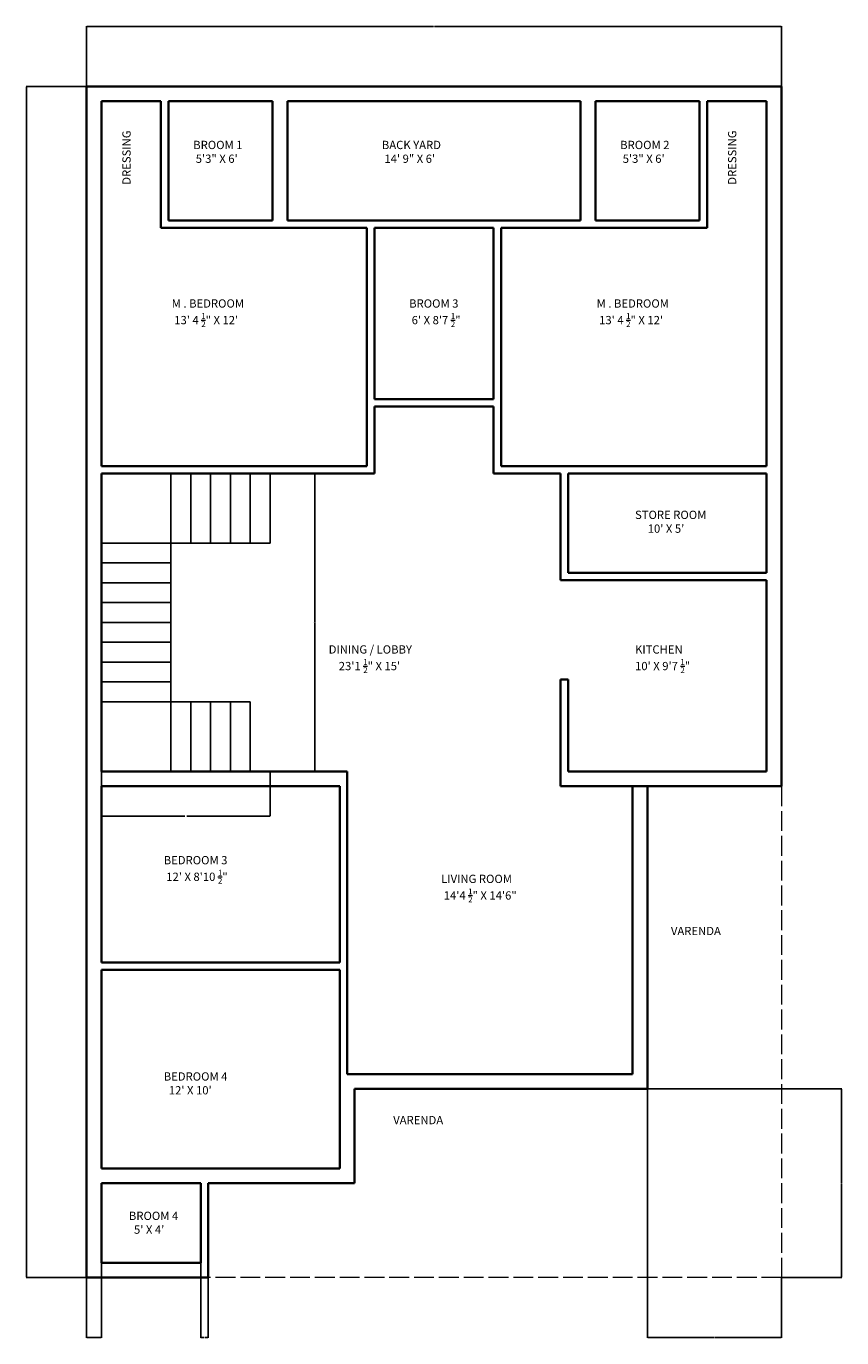
# Model space of a CAD drawing. Units: inches. Extents: x 1159 to 4240, y 1112 to 2085.
# Tile 13 of 13: x 3747 to 4240, y 1211 to 2004. Entities that reach past the tile are written whole.
import ezdxf

# ---------------------------------------------------------------- set-up
doc = ezdxf.new("R2010")
doc.units = ezdxf.units.IN
doc.linetypes.add('ACAD_ISO02W100', pattern=[15, 12, -3])
for name, color, linetype, lineweight in [('A-ANNO-DIMS', 2, 'Continuous', 18), ('A-AREA-IDEN', 30, 'Continuous', 18), ('A-FLOR-EDGE', 1, 'ACAD_ISO02W100', 18), ('STAIRCASE', 150, 'Continuous', 25), ('WALL', 7, 'Continuous', 35)]:
    doc.layers.add(name, color=color, linetype=linetype, lineweight=lineweight)
doc.styles.get("Standard").update_dxf_attribs({"font": 'arial.ttf'})
doc.dimstyles.get("Standard").update_dxf_attribs({"dimtxt": 0.18, "dimasz": 0.18, "dimexe": 0.18, "dimexo": 0.0625, "dimgap": 0.09, "dimtad": 0, "dimtih": 1, "dimtoh": 1, "dimdec": 4, "dimzin": 0, "dimdsep": 46, "dimtxsty": 'Standard', "dimcen": 0.09, "dimadec": 0, "dimazin": 0, "dimtfac": 1, "dimtdec": 4, "dimtofl": 0, "dimtmove": 0, "dimatfit": 3, "dimfxl": 1, "dimtolj": 1, "dimtzin": 0, "dimarcsym": 0})

# ---------------------------------------------------------------- blocks, each defined once
blk = doc.blocks.new('HOUSE-35x60-WALL-LAYOUT')
for p, q in [((0, 0), (0, 720)), ((0, 720), (420, 720)), ((420, 720), (420, 297)), ((9, 711), (45, 711)), ((9, 634.5), (9, 711)), ((45, 634.5), (45, 711)), ((49.5, 639), (49.5, 711)), ((49.5, 711), (112.5, 711)), ((112.5, 639), (112.5, 711)), ((121.5, 639), (121.5, 711)), ((121.5, 711), (298.5, 711)), ((298.5, 711), (298.5, 639)), ((307.5, 711), (307.5, 639)), ((307.5, 711), (370.5, 711)), ((370.5, 711), (370.5, 639)), ((375, 711), (375, 634.5)), ((375, 711), (411, 711)), ((411, 711), (411, 634.5)), ((9, 490.5), (9, 634.5)), ((45, 634.5), (169.5, 634.5)), ((49.5, 639), (112.5, 639)), ((121.5, 639), (298.5, 639)), ((169.5, 634.5), (169.5, 490.5)), ((174, 634.5), (174, 531)), ((174, 634.5), (246, 634.5)), ((246, 634.5), (246, 531)), ((250.5, 634.5), (250.5, 490.5)), ((250.5, 634.5), (375, 634.5)), ((307.5, 639), (370.5, 639)), ((411, 634.5), (411, 490.5)), ((174, 531), (246, 531)), ((174, 526.5), (246, 526.5)), ((174, 526.5), (174, 486)), ((246, 526.5), (246, 486)), ((9, 490.5), (169.5, 490.5)), ((9, 486), (174, 486)), ((9, 306), (9, 486)), ((246, 486), (286.5, 486)), ((250.5, 490.5), (411, 490.5)), ((286.5, 486), (286.5, 421.5)), ((291, 486), (291, 426)), ((291, 486), (411, 486)), ((411, 486), (411, 426)), ((291, 421.5), (286.5, 421.5)), ((291, 426), (411, 426)), ((291, 421.5), (411, 421.5)), ((411, 421.5), (411, 306)), ((291, 361.5), (286.5, 361.5)), ((286.5, 361.5), (286.5, 297)), ((291, 361.5), (291, 306)), ((9, 306), (157.5, 306)), ((157.5, 190.5), (157.5, 306)), ((291, 306), (411, 306)), ((9, 297), (153, 297)), ((9, 190.5), (9, 297)), ((153, 190.5), (153, 297)), ((286.5, 297), (420, 297)), ((330, 297), (330, 123)), ((339, 297), (339, 114)), ((153, 190.5), (9, 190.5)), ((157.5, 123), (157.5, 190.5)), ((9, 66), (9, 186)), ((153, 186), (9, 186)), ((153, 66), (153, 186)), ((330, 123), (157.5, 123)), ((162, 57), (162, 114)), ((339, 114), (162, 114)), ((153, 66), (9, 66)), ((9, 9), (9, 57)), ((69, 57), (9, 57)), ((69, 9), (69, 57)), ((162, 57), (73.5, 57)), ((73.5, 0), (73.5, 57)), ((69, 9), (9, 9)), ((0, 0), (73.5, 0))]:
    blk.add_line(p, q)
blk = doc.blocks.new('STAIR-THREE-FLIGHT')
for p, q in [((42, 138), (42, 180)), ((54, 138), (54, 180)), ((66, 138), (66, 180)), ((78, 138), (78, 180)), ((90, 138), (90, 180)), ((102, 138), (102, 180)), ((0, 138), (42, 138)), ((102, 138), (42, 138)), ((42, 138), (42, 42)), ((0, 126), (42, 126)), ((0, 114), (42, 114)), ((0, 102), (42, 102)), ((0, 90), (42, 90)), ((0, 78), (42, 78)), ((0, 66), (42, 66)), ((0, 54), (42, 54)), ((0, 42), (42, 42)), ((42, 0), (42, 42)), ((42, 42), (90, 42)), ((54, 0), (54, 42)), ((66, 0), (66, 42)), ((78, 0), (78, 42)), ((90, 0), (90, 42))]:
    blk.add_line(p, q)
blk = doc.blocks.new('*D8')
at = {"layer": 'A-ANNO-DIMS', "color": 0, "lineweight": -2, "transparency": 16777216}
for p, q in [((3894.92, 1733.7), (3922.04, 1733.7)), ((3921.86, 1733.52), (3921.86, 1643.89)), ((3921.86, 1553.88), (3921.86, 1643.52)), ((3894.92, 1553.7), (3922.04, 1553.7))]:
    blk.add_line(p, q, dxfattribs=at)
at = {"layer": 'A-ANNO-DIMS', "color": 0, "lineweight": 100, "transparency": 16777216}
for points in [[(3921.83, 1733.52), (3921.89, 1733.52), (3921.86, 1733.7)], [(3921.83, 1553.88), (3921.89, 1553.88), (3921.86, 1553.7)]]:
    blk.add_solid(points, dxfattribs=at)
at = {"layer": 'Defpoints', "color": 0, "lineweight": 100, "transparency": 16777216}
for p in [(3894.86, 1733.7), (3921.86, 1733.7), (3894.86, 1553.7)]:
    blk.add_point(p, dxfattribs=at)
at = {"layer": 'A-ANNO-DIMS', "color": 0, "transparency": 16777216, "insert": (3921.86, 1643.7), "char_height": 0.18, "attachment_point": 5}
blk.add_mtext('\\A1;STAIR 180 TYP.', dxfattribs=at)
blk = doc.blocks.new('*D9')
at = {"layer": 'A-ANNO-DIMS', "color": 0, "lineweight": -2, "transparency": 16777216}
for p, q in [((3792.86, 1553.64), (3792.86, 1526.52)), ((3894.86, 1553.64), (3894.86, 1526.52)), ((3793.04, 1526.7), (3843.27, 1526.7)), ((3894.68, 1526.7), (3844.45, 1526.7))]:
    blk.add_line(p, q, dxfattribs=at)
at = {"layer": 'A-ANNO-DIMS', "color": 0, "lineweight": 100, "transparency": 16777216}
for points in [[(3793.04, 1526.73), (3793.04, 1526.67), (3792.86, 1526.7)], [(3894.68, 1526.73), (3894.68, 1526.67), (3894.86, 1526.7)]]:
    blk.add_solid(points, dxfattribs=at)
at = {"layer": 'Defpoints', "color": 0, "lineweight": 100, "transparency": 16777216}
for p in [(3792.86, 1553.7), (3894.86, 1553.7), (3894.86, 1526.7)]:
    blk.add_point(p, dxfattribs=at)
at = {"layer": 'A-ANNO-DIMS', "color": 0, "transparency": 16777216, "insert": (3843.86, 1526.7), "char_height": 0.18, "attachment_point": 5}
blk.add_mtext('\\A1;102 TYP.', dxfattribs=at)
blk = doc.blocks.new('*D16')
at = {"layer": 'A-ANNO-DIMS', "color": 0, "lineweight": -2, "transparency": 16777216}
for p, q in [((3783.86, 1967.76), (3783.86, 2004.08)), ((3784.04, 2003.9), (3993.56, 2003.9)), ((4203.68, 2003.9), (3994.15, 2003.9)), ((4203.86, 1967.76), (4203.86, 2004.08))]:
    blk.add_line(p, q, dxfattribs=at)
at = {"layer": 'A-ANNO-DIMS', "color": 0, "lineweight": 100, "transparency": 16777216}
for points in [[(3784.04, 2003.93), (3784.04, 2003.87), (3783.86, 2003.9)], [(4203.68, 2003.93), (4203.68, 2003.87), (4203.86, 2003.9)]]:
    blk.add_solid(points, dxfattribs=at)
at = {"layer": 'Defpoints', "color": 0, "lineweight": 100, "transparency": 16777216}
for p in [(4203.86, 2003.9), (3783.86, 1967.7), (4203.86, 1967.7)]:
    blk.add_point(p, dxfattribs=at)
at = {"layer": 'A-ANNO-DIMS', "color": 0, "transparency": 16777216, "insert": (3993.86, 2003.9), "char_height": 0.18, "attachment_point": 5}
blk.add_mtext('\\A1;420', dxfattribs=at)
blk = doc.blocks.new('*D17')
at = {"layer": 'A-ANNO-DIMS', "color": 0, "lineweight": -2, "transparency": 16777216}
for p, q in [((3783.79, 1967.7), (3747.48, 1967.7)), ((3747.66, 1967.52), (3747.66, 1607.88)), ((3747.66, 1247.88), (3747.66, 1607.52)), ((3783.79, 1247.7), (3747.48, 1247.7))]:
    blk.add_line(p, q, dxfattribs=at)
at = {"layer": 'A-ANNO-DIMS', "color": 0, "lineweight": 100, "transparency": 16777216}
for points in [[(3747.63, 1967.52), (3747.69, 1967.52), (3747.66, 1967.7)], [(3747.63, 1247.88), (3747.69, 1247.88), (3747.66, 1247.7)]]:
    blk.add_solid(points, dxfattribs=at)
at = {"layer": 'Defpoints', "color": 0, "lineweight": 100, "transparency": 16777216}
for p in [(3747.66, 1967.7), (3783.86, 1967.7), (3783.86, 1247.7)]:
    blk.add_point(p, dxfattribs=at)
at = {"layer": 'A-ANNO-DIMS', "color": 0, "transparency": 16777216, "insert": (3747.66, 1607.7), "char_height": 0.18, "attachment_point": 5}
blk.add_mtext('\\A1;720', dxfattribs=at)
blk = doc.blocks.new('*D18')
at = {"layer": 'A-ANNO-DIMS', "color": 0, "lineweight": -2, "transparency": 16777216}
for p, q in [((3792.86, 1256.64), (3792.86, 1211.32)), ((3783.86, 1247.64), (3783.86, 1211.32)), ((3784.04, 1211.5), (3788.21, 1211.5)), ((3792.68, 1211.5), (3788.51, 1211.5))]:
    blk.add_line(p, q, dxfattribs=at)
at = {"layer": 'A-ANNO-DIMS', "color": 0, "lineweight": 100, "transparency": 16777216}
for points in [[(3784.04, 1211.53), (3784.04, 1211.47), (3783.86, 1211.5)], [(3792.68, 1211.53), (3792.68, 1211.47), (3792.86, 1211.5)]]:
    blk.add_solid(points, dxfattribs=at)
at = {"layer": 'Defpoints', "color": 0, "lineweight": 100, "transparency": 16777216}
for p in [(3792.86, 1256.7), (3783.86, 1247.7), (3792.86, 1211.5)]:
    blk.add_point(p, dxfattribs=at)
at = {"layer": 'A-ANNO-DIMS', "color": 0, "transparency": 16777216, "insert": (3788.36, 1211.5), "char_height": 0.18, "attachment_point": 5}
blk.add_mtext('\\A1;9', dxfattribs=at)
blk = doc.blocks.new('*D19')
at = {"layer": 'A-ANNO-DIMS', "color": 0, "lineweight": -2, "transparency": 16777216}
for p, q in [((3852.86, 1256.64), (3852.86, 1211.32)), ((3857.36, 1247.64), (3857.36, 1211.32)), ((3853.04, 1211.5), (3854.85, 1211.5)), ((3857.18, 1211.5), (3855.36, 1211.5))]:
    blk.add_line(p, q, dxfattribs=at)
at = {"layer": 'A-ANNO-DIMS', "color": 0, "lineweight": 100, "transparency": 16777216}
for points in [[(3853.04, 1211.53), (3853.04, 1211.47), (3852.86, 1211.5)], [(3857.18, 1211.53), (3857.18, 1211.47), (3857.36, 1211.5)]]:
    blk.add_solid(points, dxfattribs=at)
at = {"layer": 'Defpoints', "color": 0, "lineweight": 100, "transparency": 16777216}
for p in [(3852.86, 1256.7), (3857.36, 1247.7), (3857.36, 1211.5)]:
    blk.add_point(p, dxfattribs=at)
at = {"layer": 'A-ANNO-DIMS', "color": 0, "transparency": 16777216, "insert": (3855.11, 1211.5), "char_height": 0.18, "attachment_point": 5}
blk.add_mtext('\\A1;4.5', dxfattribs=at)
blk = doc.blocks.new('*D20')
at = {"layer": 'A-ANNO-DIMS', "color": 0, "lineweight": -2, "transparency": 16777216}
for p, q in [((4122.86, 1361.64), (4122.86, 1211.32)), ((4203.86, 1247.64), (4203.86, 1211.32)), ((4123.04, 1211.5), (4163.15, 1211.5)), ((4203.68, 1211.5), (4163.56, 1211.5))]:
    blk.add_line(p, q, dxfattribs=at)
at = {"layer": 'A-ANNO-DIMS', "color": 0, "lineweight": 100, "transparency": 16777216}
for points in [[(4123.04, 1211.53), (4123.04, 1211.47), (4122.86, 1211.5)], [(4203.68, 1211.53), (4203.68, 1211.47), (4203.86, 1211.5)]]:
    blk.add_solid(points, dxfattribs=at)
at = {"layer": 'Defpoints', "color": 0, "lineweight": 100, "transparency": 16777216}
for p in [(4122.86, 1361.7), (4203.86, 1247.7), (4203.86, 1211.5)]:
    blk.add_point(p, dxfattribs=at)
at = {"layer": 'A-ANNO-DIMS', "color": 0, "transparency": 16777216, "insert": (4163.36, 1211.5), "char_height": 0.18, "attachment_point": 5}
blk.add_mtext('\\A1;81', dxfattribs=at)
blk = doc.blocks.new('*D21')
at = {"layer": 'A-ANNO-DIMS', "color": 0, "lineweight": -2, "transparency": 16777216}
for p, q in [((4122.92, 1361.7), (4240.24, 1361.7)), ((4240.06, 1361.52), (4240.06, 1304.88)), ((4240.06, 1247.88), (4240.06, 1304.52)), ((4203.92, 1247.7), (4240.24, 1247.7))]:
    blk.add_line(p, q, dxfattribs=at)
at = {"layer": 'A-ANNO-DIMS', "color": 0, "lineweight": 100, "transparency": 16777216}
for points in [[(4240.03, 1361.52), (4240.09, 1361.52), (4240.06, 1361.7)], [(4240.03, 1247.88), (4240.09, 1247.88), (4240.06, 1247.7)]]:
    blk.add_solid(points, dxfattribs=at)
at = {"layer": 'Defpoints', "color": 0, "lineweight": 100, "transparency": 16777216}
for p in [(4122.86, 1361.7), (4203.86, 1247.7), (4240.06, 1247.7)]:
    blk.add_point(p, dxfattribs=at)
at = {"layer": 'A-ANNO-DIMS', "color": 0, "transparency": 16777216, "insert": (4240.06, 1304.7), "char_height": 0.18, "attachment_point": 5}
blk.add_mtext('\\A1;114', dxfattribs=at)

msp = doc.modelspace()

# ---------------------------------------------------------------- linework, layer by layer
at = {"layer": 'A-FLOR-EDGE'}
for p, q in [((4203.856, 1544.702), (4203.856, 1247.702)), ((4203.856, 1247.702), (3857.356, 1247.702))]:
    msp.add_line(p, q, dxfattribs=at)

# ---------------------------------------------------------------- block references
at = {"layer": 'STAIRCASE'}
msp.add_blockref('STAIR-THREE-FLIGHT', (3792.857, 1553.702), dxfattribs=at)
at = {"layer": 'WALL'}
msp.add_blockref('HOUSE-35x60-WALL-LAYOUT', (3783.857, 1247.702), dxfattribs=at)

# ---------------------------------------------------------------- texts
at = {"layer": 'A-AREA-IDEN', "char_height": 5, "attachment_point": 1, "rotation": 90}
for insert in [(3805.545, 1908.276), (4171.545, 1908.276)]:
    msp.add_mtext_dynamic_manual_height_columns('\\A1;DRESSING', width=140.18614, gutter_width=12.5, heights=[0], dxfattribs=dict(at, insert=insert))
at = {"layer": 'A-AREA-IDEN', "char_height": 5, "attachment_point": 1}
for s, insert in [('\\A1;BROOM 1\\P 5\'3" X 6\'', (3848.369, 1934.831)), ('\\A1;BACK YARD\\P 14\' 9" X 6\'', (3962.356, 1934.831)), ('\\A1;BROOM 2\\P 5\'3" X 6\'', (4106.369, 1934.831)), ('\\A1;M . BEDROOM\\P 13\' 4 {\\H0.7x;\\S1/2;}" X 12\'', (3835.38, 1838.992)), ('\\A1;BROOM 3\\P 6\' X 8\'7 {\\H0.7x;\\S1/2;}"', (3978.847, 1838.992)), ('\\A1;M . BEDROOM\\P 13\' 4 {\\H0.7x;\\S1/2;}" X 12\'', (4092.121, 1838.992)), ("\\A1;STORE ROOM\\P     10' X 5'", (4115.351, 1711.241)), ('\\A1;DINING / LOBBY\\P    23\'1 {\\H0.7x;\\S1/2;}" X 15\'', (3930.201, 1629.873)), ('\\A1;KITCHEN\\P10\' X 9\'7 {\\H0.7x;\\S1/2;}"', (4115.351, 1629.873)), ('\\A1;BEDROOM 3\\P 12\' X 8\'10 {\\H0.7x;\\S1/2;}"', (3830.548, 1502.503)), ('\\A1;LIVING ROOM\\P 14\'4 {\\H0.7x;\\S1/2;}" X 14\'6"', (3998.193, 1491.215)), ('\\A1;VARENDA', (4137.021, 1459.712)), ("\\A1;BEDROOM 4\\P  12' X 10'", (3830.548, 1371.76)), ('\\A1;VARENDA', (3969.214, 1345.387)), ("\\A1;BROOM 4 \\P  5' X 4'", (3809.503, 1287.528))]:
    msp.add_mtext_dynamic_manual_height_columns(s, width=140.18614, gutter_width=12.5, heights=[0], dxfattribs=dict(at, insert=insert))

# ---------------------------------------------------------------- dimensions: what is measured, and where the dimension line sits
at = {"layer": 'A-ANNO-DIMS'}
for base, p1, p2, override, picture, middle in [((4203.856, 2003.902), (3783.856, 1967.702), (4203.856, 1967.702), {"dimdec": 0, "dimlfac": 1, "dimrnd": 0, "dimzin": 0, "dimdsep": 46, "dimlunit": 2}, '*D16', (3993.856, 2003.902)), ((4203.856, 1211.502), (4122.856, 1361.702), (4203.856, 1247.702), {"dimdec": 0, "dimlfac": 1, "dimrnd": 0, "dimzin": 0, "dimdsep": 46, "dimlunit": 2}, '*D20', (4163.356, 1211.502)), ((3792.856, 1211.502), (3783.856, 1247.702), (3792.856, 1256.702), {"dimdec": 0, "dimlfac": 1, "dimrnd": 0, "dimzin": 0, "dimdsep": 46, "dimlunit": 2}, '*D18', (3788.356, 1211.502)), ((3857.356, 1211.502), (3852.856, 1256.702), (3857.356, 1247.702), {"dimdec": 1, "dimlfac": 1, "dimrnd": 0, "dimzin": 0, "dimdsep": 46, "dimlunit": 2}, '*D19', (3855.106, 1211.502))]:
    dim = msp.add_linear_dim(base=base, p1=p1, p2=p2, dimstyle='Standard', override=override, dxfattribs=at)
    dim.commit()
    dim.dimension.update_dxf_attribs({"geometry": picture, "text_midpoint": middle})
for base, p1, p2, picture, middle in [((3747.656, 1967.702), (3783.856, 1247.702), (3783.856, 1967.702), '*D17', (3747.656, 1607.702)), ((4240.056, 1247.702), (4122.856, 1361.702), (4203.856, 1247.702), '*D21', (4240.056, 1304.702))]:
    dim = msp.add_linear_dim(base=base, p1=p1, p2=p2, angle=90, dimstyle='Standard', override={"dimdec": 0, "dimlfac": 1, "dimrnd": 0, "dimzin": 0, "dimdsep": 46, "dimlunit": 2}, dxfattribs=at)
    dim.commit()
    dim.dimension.update_dxf_attribs({"geometry": picture, "text_midpoint": middle})
dim = msp.add_linear_dim(base=(3921.856, 1733.702), p1=(3894.856, 1553.702), p2=(3894.856, 1733.702), angle=90, text='STAIR <> TYP.', dimstyle='Standard', override={"dimdec": 0, "dimlfac": 1, "dimrnd": 0, "dimzin": 0, "dimdsep": 46, "dimlunit": 2}, dxfattribs=at)
dim.commit()
dim.dimension.update_dxf_attribs({"geometry": '*D8', "text_midpoint": (3921.856, 1643.702)})
dim = msp.add_linear_dim(base=(3894.856, 1526.702), p1=(3792.856, 1553.702), p2=(3894.856, 1553.702), text='<> TYP.', dimstyle='Standard', override={"dimdec": 0, "dimlfac": 1, "dimrnd": 0, "dimzin": 0, "dimdsep": 46, "dimlunit": 2}, dxfattribs=at)
dim.commit()
dim.dimension.update_dxf_attribs({"geometry": '*D9', "text_midpoint": (3843.856, 1526.702)})

doc.saveas('drawing.dxf')
